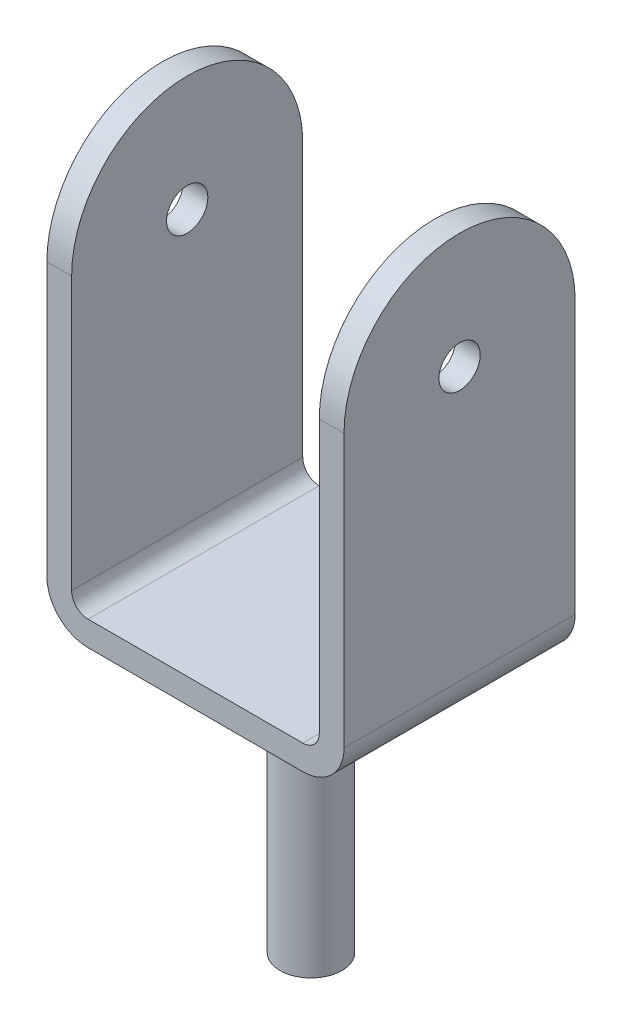
ISO-10303-21;
HEADER;
FILE_DESCRIPTION(('STEP AP214'),'2;1');
FILE_NAME('part.step','',(''),(''),'','','');
FILE_SCHEMA(('AUTOMOTIVE_DESIGN { 1 0 10303 214 1 1 1 1 }'));
ENDSEC;
DATA;
#1=APPLICATION_CONTEXT('core data for automotive mechanical design processes');
#2=APPLICATION_PROTOCOL_DEFINITION('international standard','automotive_design',2000,#1);
#3=PRODUCT_CONTEXT('',#1,'mechanical');
#4=PRODUCT('Part','Part','',(#3));
#5=PRODUCT_RELATED_PRODUCT_CATEGORY('part','',(#4));
#6=PRODUCT_DEFINITION_FORMATION('','',#4);
#7=PRODUCT_DEFINITION_CONTEXT('part definition',#1,'design');
#8=PRODUCT_DEFINITION('design','',#6,#7);
#9=PRODUCT_DEFINITION_SHAPE('','',#8);
#10=(LENGTH_UNIT() NAMED_UNIT(*) SI_UNIT(.MILLI.,.METRE.));
#11=(NAMED_UNIT(*) PLANE_ANGLE_UNIT() SI_UNIT($,.RADIAN.));
#12=(NAMED_UNIT(*) SI_UNIT($,.STERADIAN.) SOLID_ANGLE_UNIT());
#13=UNCERTAINTY_MEASURE_WITH_UNIT(LENGTH_MEASURE(1.E-05),#10,'distance_accuracy_value','');
#14=(GEOMETRIC_REPRESENTATION_CONTEXT(3) GLOBAL_UNCERTAINTY_ASSIGNED_CONTEXT((#13)) GLOBAL_UNIT_ASSIGNED_CONTEXT((#10,
#11,#12)) REPRESENTATION_CONTEXT('',''));
#15=CARTESIAN_POINT('',(0.,0.,0.));
#16=DIRECTION('',(0.,0.,1.));
#17=DIRECTION('',(1.,0.,0.));
#18=AXIS2_PLACEMENT_3D('',#15,#16,#17);
#19=CARTESIAN_POINT('',(-180.,380.,140.));
#20=DIRECTION('',(1.,0.,0.));
#21=DIRECTION('',(0.,1.,0.));
#22=AXIS2_PLACEMENT_3D('',#19,#20,#21);
#23=PLANE('',#22);
#24=CARTESIAN_POINT('',(-180.,380.,0.));
#25=DIRECTION('',(-1.,0.,0.));
#26=DIRECTION('',(0.,-1.,0.));
#27=AXIS2_PLACEMENT_3D('',#24,#25,#26);
#28=CIRCLE('',#27,25.);
#29=CARTESIAN_POINT('',(-180.,355.,0.));
#30=VERTEX_POINT('',#29);
#31=EDGE_CURVE('E328',#30,#30,#28,.T.);
#32=ORIENTED_EDGE('',*,*,#31,.F.);
#33=EDGE_LOOP('',(#32));
#34=FACE_BOUND('',#33,.T.);
#35=DIRECTION('',(0.,-1.,0.));
#36=VECTOR('',#35,1.);
#37=CARTESIAN_POINT('',(-180.,380.,140.));
#38=LINE('',#37,#36);
#39=CARTESIAN_POINT('',(-180.,380.,140.));
#40=VERTEX_POINT('',#39);
#41=CARTESIAN_POINT('',(-180.,50.,140.));
#42=VERTEX_POINT('',#41);
#43=EDGE_CURVE('E153',#40,#42,#38,.T.);
#44=ORIENTED_EDGE('',*,*,#43,.F.);
#45=CARTESIAN_POINT('',(-180.,380.,0.));
#46=DIRECTION('',(1.,0.,0.));
#47=DIRECTION('',(0.,1.,0.));
#48=AXIS2_PLACEMENT_3D('',#45,#46,#47);
#49=CIRCLE('',#48,140.);
#50=CARTESIAN_POINT('',(-180.,380.,-140.));
#51=VERTEX_POINT('',#50);
#52=EDGE_CURVE('E143',#51,#40,#49,.T.);
#53=ORIENTED_EDGE('',*,*,#52,.F.);
#54=DIRECTION('',(0.,-1.,0.));
#55=VECTOR('',#54,1.);
#56=CARTESIAN_POINT('',(-180.,380.,-140.));
#57=LINE('',#56,#55);
#58=CARTESIAN_POINT('',(-180.,50.,-140.));
#59=VERTEX_POINT('',#58);
#60=EDGE_CURVE('E130',#51,#59,#57,.T.);
#61=ORIENTED_EDGE('',*,*,#60,.T.);
#62=DIRECTION('',(0.,0.,-1.));
#63=VECTOR('',#62,1.);
#64=CARTESIAN_POINT('',(-180.,50.,140.));
#65=LINE('',#64,#63);
#66=EDGE_CURVE('E218',#59,#42,#65,.F.);
#67=ORIENTED_EDGE('',*,*,#66,.T.);
#68=EDGE_LOOP('',(#44,#53,#61,#67));
#69=FACE_BOUND('',#68,.T.);
#70=ADVANCED_FACE('F39',(#34,#69),#23,.F.);
#71=CARTESIAN_POINT('',(-180.,0.,140.));
#72=DIRECTION('',(0.,1.,0.));
#73=DIRECTION('',(-1.,0.,0.));
#74=AXIS2_PLACEMENT_3D('',#71,#72,#73);
#75=PLANE('',#74);
#76=CARTESIAN_POINT('',(0.,0.,0.));
#77=DIRECTION('',(0.,-1.,0.));
#78=DIRECTION('',(1.,0.,0.));
#79=AXIS2_PLACEMENT_3D('',#76,#77,#78);
#80=CIRCLE('',#79,37.5);
#81=CARTESIAN_POINT('',(37.5,0.,0.));
#82=VERTEX_POINT('',#81);
#83=EDGE_CURVE('E170',#82,#82,#80,.T.);
#84=ORIENTED_EDGE('',*,*,#83,.F.);
#85=EDGE_LOOP('',(#84));
#86=FACE_BOUND('',#85,.T.);
#87=DIRECTION('',(1.,0.,0.));
#88=VECTOR('',#87,1.);
#89=CARTESIAN_POINT('',(-180.,0.,-140.));
#90=LINE('',#89,#88);
#91=CARTESIAN_POINT('',(-130.,0.,-140.));
#92=VERTEX_POINT('',#91);
#93=CARTESIAN_POINT('',(130.,0.,-140.));
#94=VERTEX_POINT('',#93);
#95=EDGE_CURVE('E140',#92,#94,#90,.T.);
#96=ORIENTED_EDGE('',*,*,#95,.T.);
#97=DIRECTION('',(0.,0.,-1.));
#98=VECTOR('',#97,1.);
#99=CARTESIAN_POINT('',(130.,0.,140.));
#100=LINE('',#99,#98);
#101=CARTESIAN_POINT('',(130.,0.,140.));
#102=VERTEX_POINT('',#101);
#103=EDGE_CURVE('E208',#94,#102,#100,.F.);
#104=ORIENTED_EDGE('',*,*,#103,.T.);
#105=DIRECTION('',(1.,0.,0.));
#106=VECTOR('',#105,1.);
#107=CARTESIAN_POINT('',(-180.,0.,140.));
#108=LINE('',#107,#106);
#109=CARTESIAN_POINT('',(-130.,0.,140.));
#110=VERTEX_POINT('',#109);
#111=EDGE_CURVE('E176',#110,#102,#108,.T.);
#112=ORIENTED_EDGE('',*,*,#111,.F.);
#113=DIRECTION('',(0.,0.,-1.));
#114=VECTOR('',#113,1.);
#115=CARTESIAN_POINT('',(-130.,0.,140.));
#116=LINE('',#115,#114);
#117=EDGE_CURVE('E210',#110,#92,#116,.T.);
#118=ORIENTED_EDGE('',*,*,#117,.T.);
#119=EDGE_LOOP('',(#96,#104,#112,#118));
#120=FACE_BOUND('',#119,.T.);
#121=ADVANCED_FACE('F265',(#86,#120),#75,.F.);
#122=CARTESIAN_POINT('',(180.,0.,140.));
#123=DIRECTION('',(-1.,0.,0.));
#124=DIRECTION('',(0.,-1.,0.));
#125=AXIS2_PLACEMENT_3D('',#122,#123,#124);
#126=PLANE('',#125);
#127=CARTESIAN_POINT('',(180.,380.,0.));
#128=DIRECTION('',(-1.,0.,0.));
#129=DIRECTION('',(0.,-1.,0.));
#130=AXIS2_PLACEMENT_3D('',#127,#128,#129);
#131=CIRCLE('',#130,25.);
#132=CARTESIAN_POINT('',(180.,355.,0.));
#133=VERTEX_POINT('',#132);
#134=EDGE_CURVE('E321',#133,#133,#131,.T.);
#135=ORIENTED_EDGE('',*,*,#134,.T.);
#136=EDGE_LOOP('',(#135));
#137=FACE_BOUND('',#136,.T.);
#138=DIRECTION('',(0.,1.,0.));
#139=VECTOR('',#138,1.);
#140=CARTESIAN_POINT('',(180.,0.,-140.));
#141=LINE('',#140,#139);
#142=CARTESIAN_POINT('',(180.,50.0000000000001,-140.));
#143=VERTEX_POINT('',#142);
#144=CARTESIAN_POINT('',(180.,380.,-140.));
#145=VERTEX_POINT('',#144);
#146=EDGE_CURVE('E192',#143,#145,#141,.T.);
#147=ORIENTED_EDGE('',*,*,#146,.T.);
#148=CARTESIAN_POINT('',(180.,380.,0.));
#149=DIRECTION('',(1.,0.,0.));
#150=DIRECTION('',(0.,1.,0.));
#151=AXIS2_PLACEMENT_3D('',#148,#149,#150);
#152=CIRCLE('',#151,140.);
#153=CARTESIAN_POINT('',(180.,380.,140.));
#154=VERTEX_POINT('',#153);
#155=EDGE_CURVE('E151',#145,#154,#152,.T.);
#156=ORIENTED_EDGE('',*,*,#155,.T.);
#157=DIRECTION('',(0.,1.,0.));
#158=VECTOR('',#157,1.);
#159=CARTESIAN_POINT('',(180.,0.,140.));
#160=LINE('',#159,#158);
#161=CARTESIAN_POINT('',(180.,50.0000000000001,140.));
#162=VERTEX_POINT('',#161);
#163=EDGE_CURVE('E177',#162,#154,#160,.T.);
#164=ORIENTED_EDGE('',*,*,#163,.F.);
#165=DIRECTION('',(0.,0.,-1.));
#166=VECTOR('',#165,1.);
#167=CARTESIAN_POINT('',(180.,50.0000000000001,140.));
#168=LINE('',#167,#166);
#169=EDGE_CURVE('E167',#162,#143,#168,.T.);
#170=ORIENTED_EDGE('',*,*,#169,.T.);
#171=EDGE_LOOP('',(#147,#156,#164,#170));
#172=FACE_BOUND('',#171,.T.);
#173=ADVANCED_FACE('F253',(#137,#172),#126,.F.);
#174=CARTESIAN_POINT('',(150.,30.,140.));
#175=DIRECTION('',(1.,0.,0.));
#176=DIRECTION('',(0.,0.,-1.));
#177=AXIS2_PLACEMENT_3D('',#174,#175,#176);
#178=PLANE('',#177);
#179=CARTESIAN_POINT('',(150.,380.,0.));
#180=DIRECTION('',(1.,0.,0.));
#181=DIRECTION('',(0.,0.,-1.));
#182=AXIS2_PLACEMENT_3D('',#179,#180,#181);
#183=CIRCLE('',#182,25.);
#184=CARTESIAN_POINT('',(150.,380.,-25.));
#185=VERTEX_POINT('',#184);
#186=EDGE_CURVE('E152',#185,#185,#183,.T.);
#187=ORIENTED_EDGE('',*,*,#186,.T.);
#188=EDGE_LOOP('',(#187));
#189=FACE_BOUND('',#188,.T.);
#190=DIRECTION('',(0.,-1.,0.));
#191=VECTOR('',#190,1.);
#192=CARTESIAN_POINT('',(150.,30.,140.));
#193=LINE('',#192,#191);
#194=CARTESIAN_POINT('',(150.,380.,140.));
#195=VERTEX_POINT('',#194);
#196=CARTESIAN_POINT('',(150.,50.,140.));
#197=VERTEX_POINT('',#196);
#198=EDGE_CURVE('E182',#195,#197,#193,.T.);
#199=ORIENTED_EDGE('',*,*,#198,.F.);
#200=CARTESIAN_POINT('',(150.,380.,0.));
#201=DIRECTION('',(1.,0.,0.));
#202=DIRECTION('',(0.,1.,0.));
#203=AXIS2_PLACEMENT_3D('',#200,#201,#202);
#204=CIRCLE('',#203,140.);
#205=CARTESIAN_POINT('',(150.,380.,-140.));
#206=VERTEX_POINT('',#205);
#207=EDGE_CURVE('E156',#206,#195,#204,.T.);
#208=ORIENTED_EDGE('',*,*,#207,.F.);
#209=DIRECTION('',(0.,-1.,0.));
#210=VECTOR('',#209,1.);
#211=CARTESIAN_POINT('',(150.,30.,-140.));
#212=LINE('',#211,#210);
#213=CARTESIAN_POINT('',(150.,50.,-140.));
#214=VERTEX_POINT('',#213);
#215=EDGE_CURVE('E198',#206,#214,#212,.T.);
#216=ORIENTED_EDGE('',*,*,#215,.T.);
#217=DIRECTION('',(0.,0.,-1.));
#218=VECTOR('',#217,1.);
#219=CARTESIAN_POINT('',(150.,50.,140.));
#220=LINE('',#219,#218);
#221=EDGE_CURVE('E54',#214,#197,#220,.F.);
#222=ORIENTED_EDGE('',*,*,#221,.T.);
#223=EDGE_LOOP('',(#199,#208,#216,#222));
#224=FACE_BOUND('',#223,.T.);
#225=ADVANCED_FACE('F248',(#189,#224),#178,.F.);
#226=CARTESIAN_POINT('',(-150.,30.,140.));
#227=DIRECTION('',(0.,-1.,0.));
#228=DIRECTION('',(0.,0.,-1.));
#229=AXIS2_PLACEMENT_3D('',#226,#227,#228);
#230=PLANE('',#229);
#231=DIRECTION('',(-1.,0.,0.));
#232=VECTOR('',#231,1.);
#233=CARTESIAN_POINT('',(-150.,30.,-140.));
#234=LINE('',#233,#232);
#235=CARTESIAN_POINT('',(130.,30.,-140.));
#236=VERTEX_POINT('',#235);
#237=CARTESIAN_POINT('',(-130.,30.,-140.));
#238=VERTEX_POINT('',#237);
#239=EDGE_CURVE('E197',#236,#238,#234,.T.);
#240=ORIENTED_EDGE('',*,*,#239,.T.);
#241=DIRECTION('',(0.,0.,-1.));
#242=VECTOR('',#241,1.);
#243=CARTESIAN_POINT('',(-130.,30.,140.));
#244=LINE('',#243,#242);
#245=CARTESIAN_POINT('',(-130.,30.,140.));
#246=VERTEX_POINT('',#245);
#247=EDGE_CURVE('E225',#238,#246,#244,.F.);
#248=ORIENTED_EDGE('',*,*,#247,.T.);
#249=DIRECTION('',(-1.,0.,0.));
#250=VECTOR('',#249,1.);
#251=CARTESIAN_POINT('',(-150.,30.,140.));
#252=LINE('',#251,#250);
#253=CARTESIAN_POINT('',(130.,30.,140.));
#254=VERTEX_POINT('',#253);
#255=EDGE_CURVE('E184',#254,#246,#252,.T.);
#256=ORIENTED_EDGE('',*,*,#255,.F.);
#257=DIRECTION('',(0.,0.,-1.));
#258=VECTOR('',#257,1.);
#259=CARTESIAN_POINT('',(130.,30.,-140.));
#260=LINE('',#259,#258);
#261=EDGE_CURVE('E223',#254,#236,#260,.T.);
#262=ORIENTED_EDGE('',*,*,#261,.T.);
#263=EDGE_LOOP('',(#240,#248,#256,#262));
#264=FACE_BOUND('',#263,.T.);
#265=ADVANCED_FACE('F243',(#264),#230,.F.);
#266=CARTESIAN_POINT('',(-150.,380.,140.));
#267=DIRECTION('',(-1.,0.,0.));
#268=DIRECTION('',(0.,-1.,0.));
#269=AXIS2_PLACEMENT_3D('',#266,#267,#268);
#270=PLANE('',#269);
#271=CARTESIAN_POINT('',(-150.,380.,0.));
#272=DIRECTION('',(-1.,0.,0.));
#273=DIRECTION('',(0.,-1.,0.));
#274=AXIS2_PLACEMENT_3D('',#271,#272,#273);
#275=CIRCLE('',#274,25.);
#276=CARTESIAN_POINT('',(-150.,355.,0.));
#277=VERTEX_POINT('',#276);
#278=EDGE_CURVE('E43',#277,#277,#275,.T.);
#279=ORIENTED_EDGE('',*,*,#278,.T.);
#280=EDGE_LOOP('',(#279));
#281=FACE_BOUND('',#280,.T.);
#282=DIRECTION('',(0.,1.,0.));
#283=VECTOR('',#282,1.);
#284=CARTESIAN_POINT('',(-150.,380.,-140.));
#285=LINE('',#284,#283);
#286=CARTESIAN_POINT('',(-150.,50.,-140.));
#287=VERTEX_POINT('',#286);
#288=CARTESIAN_POINT('',(-150.,380.,-140.));
#289=VERTEX_POINT('',#288);
#290=EDGE_CURVE('E172',#287,#289,#285,.T.);
#291=ORIENTED_EDGE('',*,*,#290,.T.);
#292=CARTESIAN_POINT('',(-150.,380.,0.));
#293=DIRECTION('',(1.,0.,0.));
#294=DIRECTION('',(0.,1.,0.));
#295=AXIS2_PLACEMENT_3D('',#292,#293,#294);
#296=CIRCLE('',#295,140.);
#297=CARTESIAN_POINT('',(-150.,380.,140.));
#298=VERTEX_POINT('',#297);
#299=EDGE_CURVE('E150',#289,#298,#296,.T.);
#300=ORIENTED_EDGE('',*,*,#299,.T.);
#301=DIRECTION('',(0.,1.,0.));
#302=VECTOR('',#301,1.);
#303=CARTESIAN_POINT('',(-150.,380.,140.));
#304=LINE('',#303,#302);
#305=CARTESIAN_POINT('',(-150.,50.,140.));
#306=VERTEX_POINT('',#305);
#307=EDGE_CURVE('E171',#306,#298,#304,.T.);
#308=ORIENTED_EDGE('',*,*,#307,.F.);
#309=DIRECTION('',(0.,0.,-1.));
#310=VECTOR('',#309,1.);
#311=CARTESIAN_POINT('',(-150.,50.,-140.));
#312=LINE('',#311,#310);
#313=EDGE_CURVE('E217',#306,#287,#312,.T.);
#314=ORIENTED_EDGE('',*,*,#313,.T.);
#315=EDGE_LOOP('',(#291,#300,#308,#314));
#316=FACE_BOUND('',#315,.T.);
#317=ADVANCED_FACE('F239',(#281,#316),#270,.F.);
#318=CARTESIAN_POINT('',(0.,0.,140.));
#319=DIRECTION('',(0.,0.,-1.));
#320=DIRECTION('',(-1.,0.,0.));
#321=AXIS2_PLACEMENT_3D('',#318,#319,#320);
#322=PLANE('',#321);
#323=ORIENTED_EDGE('',*,*,#111,.T.);
#324=CARTESIAN_POINT('',(130.,50.0000000000001,140.));
#325=DIRECTION('',(0.,0.,-1.));
#326=DIRECTION('',(-1.,0.,0.));
#327=AXIS2_PLACEMENT_3D('',#324,#325,#326);
#328=CIRCLE('',#327,50.);
#329=EDGE_CURVE('E211',#102,#162,#328,.F.);
#330=ORIENTED_EDGE('',*,*,#329,.T.);
#331=ORIENTED_EDGE('',*,*,#163,.T.);
#332=DIRECTION('',(-1.,0.,0.));
#333=VECTOR('',#332,1.);
#334=CARTESIAN_POINT('',(150.,380.,140.));
#335=LINE('',#334,#333);
#336=EDGE_CURVE('E181',#154,#195,#335,.T.);
#337=ORIENTED_EDGE('',*,*,#336,.T.);
#338=ORIENTED_EDGE('',*,*,#198,.T.);
#339=CARTESIAN_POINT('',(130.,50.,140.));
#340=DIRECTION('',(0.,0.,-1.));
#341=DIRECTION('',(-1.,0.,0.));
#342=AXIS2_PLACEMENT_3D('',#339,#340,#341);
#343=CIRCLE('',#342,20.);
#344=EDGE_CURVE('E11',#197,#254,#343,.T.);
#345=ORIENTED_EDGE('',*,*,#344,.T.);
#346=ORIENTED_EDGE('',*,*,#255,.T.);
#347=CARTESIAN_POINT('',(-130.,50.,140.));
#348=DIRECTION('',(0.,0.,-1.));
#349=DIRECTION('',(-1.,0.,0.));
#350=AXIS2_PLACEMENT_3D('',#347,#348,#349);
#351=CIRCLE('',#350,20.);
#352=EDGE_CURVE('E230',#246,#306,#351,.T.);
#353=ORIENTED_EDGE('',*,*,#352,.T.);
#354=ORIENTED_EDGE('',*,*,#307,.T.);
#355=DIRECTION('',(-1.,0.,0.));
#356=VECTOR('',#355,1.);
#357=CARTESIAN_POINT('',(-180.,380.,140.));
#358=LINE('',#357,#356);
#359=EDGE_CURVE('E175',#298,#40,#358,.T.);
#360=ORIENTED_EDGE('',*,*,#359,.T.);
#361=ORIENTED_EDGE('',*,*,#43,.T.);
#362=CARTESIAN_POINT('',(-130.,50.,140.));
#363=DIRECTION('',(0.,0.,-1.));
#364=DIRECTION('',(-1.,0.,0.));
#365=AXIS2_PLACEMENT_3D('',#362,#363,#364);
#366=CIRCLE('',#365,50.);
#367=EDGE_CURVE('E215',#42,#110,#366,.F.);
#368=ORIENTED_EDGE('',*,*,#367,.T.);
#369=EDGE_LOOP('',(#323,#330,#331,#337,#338,#345,#346,#353,#354,#360,#361,#368));
#370=FACE_BOUND('',#369,.T.);
#371=ADVANCED_FACE('F234',(#370),#322,.F.);
#372=CARTESIAN_POINT('',(0.,0.,-140.));
#373=DIRECTION('',(0.,0.,-1.));
#374=DIRECTION('',(-1.,0.,0.));
#375=AXIS2_PLACEMENT_3D('',#372,#373,#374);
#376=PLANE('',#375);
#377=ORIENTED_EDGE('',*,*,#146,.F.);
#378=CARTESIAN_POINT('',(130.,50.0000000000001,-140.));
#379=DIRECTION('',(0.,0.,-1.));
#380=DIRECTION('',(-1.,0.,0.));
#381=AXIS2_PLACEMENT_3D('',#378,#379,#380);
#382=CIRCLE('',#381,50.);
#383=EDGE_CURVE('E201',#143,#94,#382,.T.);
#384=ORIENTED_EDGE('',*,*,#383,.T.);
#385=ORIENTED_EDGE('',*,*,#95,.F.);
#386=CARTESIAN_POINT('',(-130.,50.,-140.));
#387=DIRECTION('',(0.,0.,-1.));
#388=DIRECTION('',(-1.,0.,0.));
#389=AXIS2_PLACEMENT_3D('',#386,#387,#388);
#390=CIRCLE('',#389,50.);
#391=EDGE_CURVE('E131',#92,#59,#390,.T.);
#392=ORIENTED_EDGE('',*,*,#391,.T.);
#393=ORIENTED_EDGE('',*,*,#60,.F.);
#394=DIRECTION('',(-1.,0.,0.));
#395=VECTOR('',#394,1.);
#396=CARTESIAN_POINT('',(-180.,380.,-140.));
#397=LINE('',#396,#395);
#398=EDGE_CURVE('E134',#289,#51,#397,.T.);
#399=ORIENTED_EDGE('',*,*,#398,.F.);
#400=ORIENTED_EDGE('',*,*,#290,.F.);
#401=CARTESIAN_POINT('',(-130.,50.,-140.));
#402=DIRECTION('',(0.,0.,-1.));
#403=DIRECTION('',(-1.,0.,0.));
#404=AXIS2_PLACEMENT_3D('',#401,#402,#403);
#405=CIRCLE('',#404,20.);
#406=EDGE_CURVE('E227',#287,#238,#405,.F.);
#407=ORIENTED_EDGE('',*,*,#406,.T.);
#408=ORIENTED_EDGE('',*,*,#239,.F.);
#409=CARTESIAN_POINT('',(130.,50.,-140.));
#410=DIRECTION('',(0.,0.,-1.));
#411=DIRECTION('',(-1.,0.,0.));
#412=AXIS2_PLACEMENT_3D('',#409,#410,#411);
#413=CIRCLE('',#412,20.);
#414=EDGE_CURVE('E48',#236,#214,#413,.F.);
#415=ORIENTED_EDGE('',*,*,#414,.T.);
#416=ORIENTED_EDGE('',*,*,#215,.F.);
#417=DIRECTION('',(-1.,0.,0.));
#418=VECTOR('',#417,1.);
#419=CARTESIAN_POINT('',(150.,380.,-140.));
#420=LINE('',#419,#418);
#421=EDGE_CURVE('E194',#145,#206,#420,.T.);
#422=ORIENTED_EDGE('',*,*,#421,.F.);
#423=EDGE_LOOP('',(#377,#384,#385,#392,#393,#399,#400,#407,#408,#415,#416,#422));
#424=FACE_BOUND('',#423,.T.);
#425=ADVANCED_FACE('F128',(#424),#376,.T.);
#426=CARTESIAN_POINT('',(0.,-325.,0.));
#427=DIRECTION('',(0.,1.,0.));
#428=DIRECTION('',(-1.,0.,0.));
#429=AXIS2_PLACEMENT_3D('',#426,#427,#428);
#430=CYLINDRICAL_SURFACE('',#429,37.5);
#431=CARTESIAN_POINT('',(0.,-325.,0.));
#432=DIRECTION('',(0.,-1.,0.));
#433=DIRECTION('',(1.,0.,0.));
#434=AXIS2_PLACEMENT_3D('',#431,#432,#433);
#435=CIRCLE('',#434,37.5);
#436=CARTESIAN_POINT('',(37.5000000000001,-325.,0.));
#437=VERTEX_POINT('',#436);
#438=EDGE_CURVE('E149',#437,#437,#435,.T.);
#439=ORIENTED_EDGE('',*,*,#438,.F.);
#440=EDGE_LOOP('',(#439));
#441=FACE_BOUND('',#440,.T.);
#442=ORIENTED_EDGE('',*,*,#83,.T.);
#443=EDGE_LOOP('',(#442));
#444=FACE_BOUND('',#443,.T.);
#445=ADVANCED_FACE('F301',(#441,#444),#430,.T.);
#446=CARTESIAN_POINT('',(0.,-325.,0.));
#447=DIRECTION('',(0.,-1.,0.));
#448=DIRECTION('',(1.,0.,0.));
#449=AXIS2_PLACEMENT_3D('',#446,#447,#448);
#450=PLANE('',#449);
#451=ORIENTED_EDGE('',*,*,#438,.T.);
#452=EDGE_LOOP('',(#451));
#453=FACE_BOUND('',#452,.T.);
#454=ADVANCED_FACE('F277',(#453),#450,.T.);
#455=CARTESIAN_POINT('',(130.,50.0000000000001,140.));
#456=DIRECTION('',(0.,0.,-1.));
#457=DIRECTION('',(-1.,0.,0.));
#458=AXIS2_PLACEMENT_3D('',#455,#456,#457);
#459=CYLINDRICAL_SURFACE('',#458,50.);
#460=ORIENTED_EDGE('',*,*,#329,.F.);
#461=ORIENTED_EDGE('',*,*,#103,.F.);
#462=ORIENTED_EDGE('',*,*,#383,.F.);
#463=ORIENTED_EDGE('',*,*,#169,.F.);
#464=EDGE_LOOP('',(#460,#461,#462,#463));
#465=FACE_BOUND('',#464,.T.);
#466=ADVANCED_FACE('F258',(#465),#459,.T.);
#467=CARTESIAN_POINT('',(-130.,50.,140.));
#468=DIRECTION('',(0.,0.,-1.));
#469=DIRECTION('',(-1.,0.,0.));
#470=AXIS2_PLACEMENT_3D('',#467,#468,#469);
#471=CYLINDRICAL_SURFACE('',#470,50.);
#472=ORIENTED_EDGE('',*,*,#367,.F.);
#473=ORIENTED_EDGE('',*,*,#66,.F.);
#474=ORIENTED_EDGE('',*,*,#391,.F.);
#475=ORIENTED_EDGE('',*,*,#117,.F.);
#476=EDGE_LOOP('',(#472,#473,#474,#475));
#477=FACE_BOUND('',#476,.T.);
#478=ADVANCED_FACE('F267',(#477),#471,.T.);
#479=CARTESIAN_POINT('',(-130.,50.,140.));
#480=DIRECTION('',(0.,0.,1.));
#481=DIRECTION('',(1.,0.,0.));
#482=AXIS2_PLACEMENT_3D('',#479,#480,#481);
#483=CYLINDRICAL_SURFACE('',#482,20.);
#484=ORIENTED_EDGE('',*,*,#352,.F.);
#485=ORIENTED_EDGE('',*,*,#247,.F.);
#486=ORIENTED_EDGE('',*,*,#406,.F.);
#487=ORIENTED_EDGE('',*,*,#313,.F.);
#488=EDGE_LOOP('',(#484,#485,#486,#487));
#489=FACE_BOUND('',#488,.T.);
#490=ADVANCED_FACE('F241',(#489),#483,.F.);
#491=CARTESIAN_POINT('',(130.,50.,140.));
#492=DIRECTION('',(0.,0.,1.));
#493=DIRECTION('',(1.,0.,0.));
#494=AXIS2_PLACEMENT_3D('',#491,#492,#493);
#495=CYLINDRICAL_SURFACE('',#494,20.);
#496=ORIENTED_EDGE('',*,*,#344,.F.);
#497=ORIENTED_EDGE('',*,*,#221,.F.);
#498=ORIENTED_EDGE('',*,*,#414,.F.);
#499=ORIENTED_EDGE('',*,*,#261,.F.);
#500=EDGE_LOOP('',(#496,#497,#498,#499));
#501=FACE_BOUND('',#500,.T.);
#502=ADVANCED_FACE('F41',(#501),#495,.F.);
#503=CARTESIAN_POINT('',(150.,380.,0.));
#504=DIRECTION('',(1.,0.,0.));
#505=DIRECTION('',(0.,1.,0.));
#506=AXIS2_PLACEMENT_3D('',#503,#504,#505);
#507=CYLINDRICAL_SURFACE('',#506,140.);
#508=ORIENTED_EDGE('',*,*,#207,.T.);
#509=ORIENTED_EDGE('',*,*,#336,.F.);
#510=ORIENTED_EDGE('',*,*,#155,.F.);
#511=ORIENTED_EDGE('',*,*,#421,.T.);
#512=EDGE_LOOP('',(#508,#509,#510,#511));
#513=FACE_BOUND('',#512,.T.);
#514=ADVANCED_FACE('F252',(#513),#507,.T.);
#515=CARTESIAN_POINT('',(-150.,380.,0.));
#516=DIRECTION('',(-1.,0.,0.));
#517=DIRECTION('',(0.,-1.,0.));
#518=AXIS2_PLACEMENT_3D('',#515,#516,#517);
#519=CYLINDRICAL_SURFACE('',#518,140.);
#520=ORIENTED_EDGE('',*,*,#52,.T.);
#521=ORIENTED_EDGE('',*,*,#359,.F.);
#522=ORIENTED_EDGE('',*,*,#299,.F.);
#523=ORIENTED_EDGE('',*,*,#398,.T.);
#524=EDGE_LOOP('',(#520,#521,#522,#523));
#525=FACE_BOUND('',#524,.T.);
#526=ADVANCED_FACE('F141',(#525),#519,.T.);
#527=CARTESIAN_POINT('',(180.,380.,0.));
#528=DIRECTION('',(-1.,0.,0.));
#529=DIRECTION('',(0.,-1.,0.));
#530=AXIS2_PLACEMENT_3D('',#527,#528,#529);
#531=CYLINDRICAL_SURFACE('',#530,25.);
#532=ORIENTED_EDGE('',*,*,#31,.T.);
#533=EDGE_LOOP('',(#532));
#534=FACE_BOUND('',#533,.T.);
#535=ORIENTED_EDGE('',*,*,#278,.F.);
#536=EDGE_LOOP('',(#535));
#537=FACE_BOUND('',#536,.T.);
#538=ADVANCED_FACE('F312',(#534,#537),#531,.F.);
#539=ORIENTED_EDGE('',*,*,#134,.F.);
#540=EDGE_LOOP('',(#539));
#541=FACE_BOUND('',#540,.T.);
#542=ORIENTED_EDGE('',*,*,#186,.F.);
#543=EDGE_LOOP('',(#542));
#544=FACE_BOUND('',#543,.T.);
#545=ADVANCED_FACE('F313',(#541,#544),#531,.F.);
#546=CLOSED_SHELL('',(#70,#121,#173,#225,#265,#317,#371,#425,#445,#454,#466,#478,#490,#502,#514,
#526,#538,#545));
#547=MANIFOLD_SOLID_BREP('B2',#546);
#548=ADVANCED_BREP_SHAPE_REPRESENTATION('',(#18,#547),#14);
#549=SHAPE_DEFINITION_REPRESENTATION(#9,#548);
ENDSEC;
END-ISO-10303-21;
